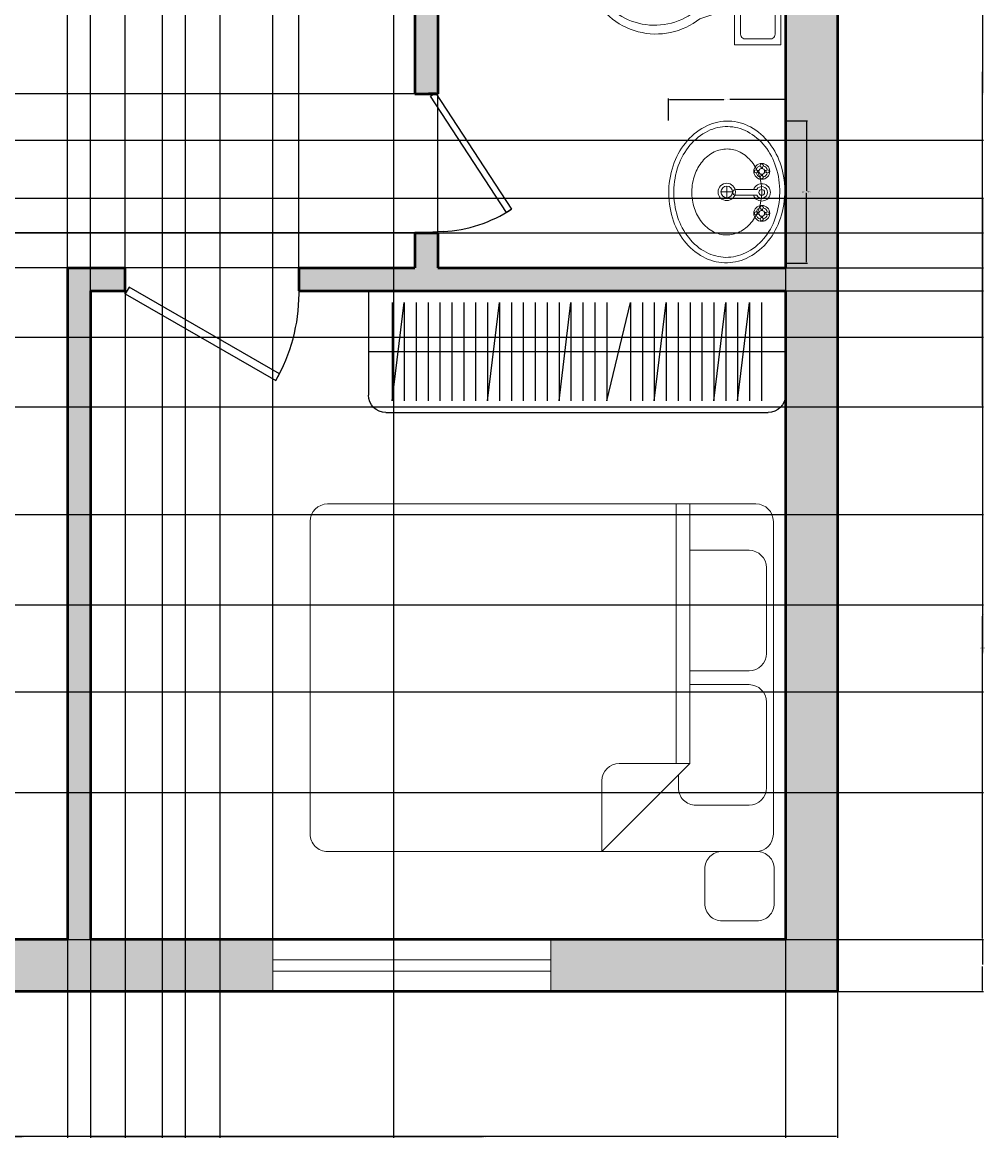
# Model space of a CAD drawing. Units: inches. Extents: x 3439 to 3988, y 1915 to 2284.
# Tile 5 of 7: x 3822 to 3988, y 1915 to 2108. Entities that reach past the tile are written whole.
import ezdxf

# ---------------------------------------------------------------- set-up
doc = ezdxf.new("R2010")
doc.units = ezdxf.units.IN
for name, color, linetype, lineweight in [('A-ANNO-DIMS', 2, 'Continuous', 18), ('A-DOOR', 3, 'Continuous', 25), ('A-FLOR-CASE', 8, 'Continuous', 25), ('A-FLOR-FIXT', 9, 'Continuous', 18), ('A-FURN', 9, 'Continuous', 18), ('A-GLAZ', 4, 'Continuous', 18), ('A-WALL', 7, 'Continuous', 50)]:
    doc.layers.add(name, color=color, linetype=linetype, lineweight=lineweight)
doc.layers.add('A-WALL-PATT', color=18, linetype='Continuous', lineweight=13, true_color=0x000000)
doc.styles.get("Standard").update_dxf_attribs({"font": 'arial.ttf'})
doc.dimstyles.get("Standard").update_dxf_attribs({"dimtxt": 0.18, "dimasz": 0.18, "dimexe": 0.18, "dimexo": 0.0625, "dimgap": 0.09, "dimtad": 0, "dimtih": 1, "dimtoh": 1, "dimdec": 4, "dimzin": 0, "dimdsep": 46, "dimtxsty": 'Standard', "dimcen": 0.09, "dimadec": 0, "dimazin": 0, "dimtfac": 1, "dimtdec": 4, "dimtofl": 0, "dimtmove": 0, "dimatfit": 3, "dimfxl": 1, "dimtolj": 1, "dimtzin": 0, "dimarcsym": 0})

# ---------------------------------------------------------------- blocks, each defined once
blk = doc.blocks.new('*U5')
for p, q in [((0, 0), (0, 6)), ((40, 0), (40, 6))]:
    blk.add_line(p, q)
blk.add_lwpolyline([(0, 0), (34.64, -20), (35.52, -18.48), (0.87, 1.52)], close=True)
blk.add_arc((0, 0), 40, 330, 0)
blk = doc.blocks.new('*U4')
for p, q in [((0, 0), (0, -6)), ((40, 0), (40, -6))]:
    blk.add_line(p, q)
blk.add_lwpolyline([(0, 0), (34.64, 20), (35.52, 18.48), (0.87, -1.52)], close=True)
blk.add_arc((0, 0), 40, 0, 30)
blk = doc.blocks.new('Toilet - top')
for p, q in [((9.5, -6), (9.5, -2)), ((-10, -8.5), (-8, -8.5)), ((-10, -9.5), (-10, -8.5)), ((-7, -9.5), (-10, -9.5)), ((-8, -8.5), (-8, -8)), ((-7, -8), (-7, -9.5)), ((-4, -8), (-6, -14)), ((4, -8), (6, -14)), ((4, -14), (-4, -14))]:
    blk.add_line(p, q)
blk.add_lwpolyline([(10.5, -8), (10.5, 0), (-10.5, 0), (-10.5, -8)], close=True)
for points in [[(8.5, -1), (-8.5, -1)], [(-9.5, -2), (-9.5, -6)], [(-8.5, -7), (8.5, -7)]]:
    blk.add_lwpolyline(points)
for centre, radius, start, end in [((-8.62, -1.88), 0.884, 81.8699, 188.1301), ((8.62, -1.88), 0.884, 351.8699, 98.1301), ((-8.62, -6.12), 0.884, 171.8699, 278.1301), ((8.62, -6.12), 0.884, 261.8699, 8.1301), ((3.52, -21.58), 12.17, 141.4691, 247.9714), ((4.2, -21.82), 11.33, 136.3677, 238.9468), ((-3.52, -21.58), 12.17, 292.0284, 38.5307), ((-4.2, -21.82), 11.33, 301.053, 43.6321), ((0, -27.88), 4, 245.7318, 294.2682), ((0, -29), 4, 254.8605, 285.1395)]:
    blk.add_arc(centre, radius, start, end)
blk = doc.blocks.new('Bed - Queen')
for p, q in [((3, 0), (56.99999, 0)), ((10.99999, -1.2), (25.79998, -1.2)), ((34.19999, -1.2), (48.99999, -1.2)), ((0, -77.00003), (0, -3)), ((59.99999, -3), (59.99999, -77.00003)), ((7.99999, -14.4), (7.99999, -4.2)), ((28.79998, -4.2), (28.79998, -14.4)), ((31.19999, -14.4), (31.19999, -4.2)), ((51.99999, -4.2), (51.99999, -13.4)), ((0, -14.4), (44.8, -14.4)), ((59.99999, -29.6), (44.8, -14.4)), ((44.8, -14.4), (44.8, -26.6)), ((44.8, -16.8), (0, -16.8)), ((48.99999, -16.4), (46.79936, -16.4)), ((47.8, -29.6), (59.99999, -29.6)), ((56.99999, -80.00003), (3, -80.00003))]:
    blk.add_line(p, q)
for centre, start, end in [((3, -3), 90, 180), ((56.99999, -3), 0, 90), ((10.99999, -4.2), 90, 180), ((25.79998, -4.2), 0, 90), ((34.19999, -4.2), 90, 180), ((48.99999, -4.2), 0, 90), ((48.99999, -13.4), 270, 0), ((47.8, -26.6), 180, 270), ((3, -77.00003), 180, 270), ((56.99999, -77.00003), 270, 0)]:
    blk.add_arc(centre, 3, start, end)
blk = doc.blocks.new('Sink - Oval top')
for p, q in [((-1, 0), (1, 0)), ((0, 1), (0, -1))]:
    blk.add_line(p, q)
for points in [[(-12.23, 0.39, 0.117634), (-11.46, -3.36, 0.104469), (-8.88, -6.8, 0.090016), (-5.08, -9.07, 0.08192), (-0.32, -10.02, 0.08192), (4.49, -9.38, 0.090016), (8.42, -7.36, 0.104469), (11.22, -4.09, 0.117634), (12.23, -0.39, 0.117634), (11.46, 3.36, 0.104469), (8.88, 6.8, 0.090016), (5.08, 9.07, 0.08192), (0.32, 10.02, 0.08192), (-4.49, 9.38, 0.090016), (-8.42, 7.36, 0.104469), (-11.22, 4.09, 0.117634)], [(-11.29, 0.16, 0.118622), (-10.52, -3.25, 0.104678), (-8.07, -6.36, 0.089562), (-4.54, -8.37, 0.081185), (-0.13, -9.15, 0.081185), (4.3, -8.49, 0.089562), (7.89, -6.58, 0.104678), (10.42, -3.55, 0.118622), (11.29, -0.16, 0.118622), (10.52, 3.25, 0.104678), (8.07, 6.36, 0.089562), (4.54, 8.37, 0.081185), (0.13, 9.15, 0.081185), (-4.3, 8.49, 0.089562), (-7.89, 6.58, 0.104678), (-10.42, 3.55, 0.118622)], [(-7.42, 0.08, 0.118283), (-6.91, -2.17, 0.104607), (-5.29, -4.21, 0.089718), (-2.97, -5.53, 0.081436), (-0.07, -6.04, 0.081436), (2.84, -5.59, 0.089718), (5.2, -4.33, 0.104607), (6.86, -2.32, 0.118283), (7.42, -0.08, 0.118283), (6.91, 2.17, 0.104607), (5.29, 4.21, 0.089718), (2.97, 5.53, 0.081436), (0.07, 6.04, 0.081436), (-2.84, 5.59, 0.089718), (-5.2, 4.33, 0.104607), (-6.86, 2.32, 0.118283)]]:
    blk.add_lwpolyline(points, format="xyb", close=True)
for radius in [1.5, 1]:
    blk.add_circle((0, 0), radius)
blk = doc.blocks.new('Faucet - Bathroom top')
for p, q in [((-4.107, 0.125), (-4.375, 0.125)), ((-3.75, 0.4788), (-3.75, 0.75)), ((-3.5, 0.482), (-3.5, 0.75)), ((-3.1461, 0.125), (-2.875, 0.125)), ((3.143, 0.125), (2.875, 0.125)), ((3.5, 0.4788), (3.5, 0.75)), ((3.75, 0.482), (3.75, 0.75)), ((4.1039, 0.125), (4.375, 0.125)), ((-4.1039, -0.125), (-4.375, -0.125)), ((-3.75, -0.4821), (-3.75, -0.75)), ((-3.5, -0.4789), (-3.5, -0.75)), ((-3.143, -0.125), (-2.875, -0.125)), ((-0.5, -0.8639), (-0.5, -4.5)), ((0.5, -4.5), (0.5, -0.8631)), ((3.1461, -0.125), (2.875, -0.125)), ((3.5, -0.4821), (3.5, -0.75)), ((3.75, -0.4789), (3.75, -0.75)), ((4.107, -0.125), (4.375, -0.125))]:
    blk.add_line(p, q)
for centre, radius in [((-3.625, 0), 1.375), ((-4.625, 0), 0.2795), ((-3.625, 0), 0.5), ((-3.625, 1), 0.2795), ((-2.625, 0), 0.2795), ((0, 0), 0.5), ((3.625, 0), 1.375), ((2.625, 0), 0.2795), ((3.625, 0), 0.5), ((3.625, 1), 0.2795), ((4.625, 0), 0.2795), ((-3.625, -1), 0.2795), ((3.625, -1), 0.2795)]:
    blk.add_circle(centre, radius)
for centre, radius, start, end in [((-3.625, 0), 1, 105.2407, 164.2093), ((-3.625, 0), 1, 16.44125, 74.07887), ((0, 0), 1.5, 289.6514, 250.3603), ((0, 0), 1, 300.3431, 239.7554), ((3.625, 0), 1, 106.12, 164.0884), ((3.625, 0), 1, 16.23422, 73.90469), ((-3.625, 0), 1, 196.2342, 253.9047), ((-3.625, 0), 1, 286.12, 344.0884), ((3.625, 0), 1, 196.4413, 254.0789), ((3.625, 0), 1, 285.2407, 344.2093), ((0, -4.5), 0.5, 180, 0)]:
    blk.add_arc(centre, radius, start, end)
blk = doc.blocks.new('WINDOW-GLASS-48IN')
for p, q in [((0, 2), (48, 2)), ((0, 0), (48, 0))]:
    blk.add_line(p, q)
blk = doc.blocks.new('WARDROBE-72IN')
for p, q in [((3, 21), (69, 21)), ((0, 0), (0, 18)), ((4.11, 2), (4.11, 19)), ((4.11, 19), (6.17, 2)), ((6.17, 2), (6.17, 19)), ((8.23, 2), (8.23, 19)), ((10.28, 2), (10.28, 19)), ((12.34, 2), (12.34, 19)), ((14.4, 2), (14.4, 19)), ((16.45, 2), (16.45, 19)), ((18.51, 2), (18.51, 19)), ((20.57, 2), (20.57, 19)), ((20.57, 19), (22.62, 2)), ((22.62, 2), (22.62, 19)), ((24.68, 2), (24.68, 19)), ((26.74, 2), (26.74, 19)), ((28.79, 2), (28.79, 19)), ((30.85, 2), (30.85, 19)), ((32.91, 2), (32.91, 19)), ((32.91, 19), (34.97, 2)), ((34.97, 2), (34.97, 19)), ((37.02, 2), (37.02, 19)), ((39.08, 2), (39.08, 19)), ((41.14, 2), (41.14, 19)), ((41.14, 19), (45.25, 2)), ((45.25, 2), (45.25, 19)), ((47.31, 2), (47.31, 19)), ((49.36, 2), (49.36, 19)), ((49.36, 19), (51.42, 2)), ((51.42, 2), (51.42, 19)), ((53.48, 2), (53.48, 19)), ((55.53, 2), (55.53, 19)), ((57.59, 2), (57.59, 19)), ((59.65, 2), (59.65, 19)), ((59.65, 19), (61.7, 2)), ((61.7, 2), (61.7, 19)), ((63.76, 2), (63.76, 19)), ((63.76, 19), (65.82, 2)), ((65.82, 2), (65.82, 19)), ((67.87, 2), (67.87, 19)), ((72, 18), (72, 0)), ((0, 10.5), (72, 10.5)), ((72, 0), (0, 0))]:
    blk.add_line(p, q)
for centre, start, end in [((3, 18), 90, 180), ((69, 18), 0, 90)]:
    blk.add_arc(centre, 3, start, end)
blk = doc.blocks.new('NIGHTSTAND-12IN-RADIUS')
blk.add_lwpolyline([(3, 0), (9, 0, 0.414214), (12, 3), (12, 9, 0.414214), (9, 12), (3, 12, 0.414214), (0, 9), (0, 3, 0.414214)], format="xyb", close=True)
blk = doc.blocks.new('*D33')
at = {"layer": 'A-ANNO-DIMS', "color": 0, "lineweight": -2, "transparency": 16777216}
for p, q in [((3953.59, 2090.71), (3957.39, 2090.71)), ((3957.21, 2090.53), (3957.21, 2078.62)), ((3957.21, 2066.34), (3957.21, 2078.25)), ((3953.59, 2066.16), (3957.39, 2066.16))]:
    blk.add_line(p, q, dxfattribs=at)
at = {"layer": 'A-ANNO-DIMS', "color": 0, "transparency": 16777216}
for points in [[(3957.18, 2090.53), (3957.24, 2090.53), (3957.21, 2090.71)], [(3957.18, 2066.34), (3957.24, 2066.34), (3957.21, 2066.16)]]:
    blk.add_solid(points, dxfattribs=at)
at = {"layer": 'Defpoints', "color": 0, "transparency": 16777216}
for p in [(3953.53, 2090.71), (3953.53, 2066.16), (3957.21, 2066.16)]:
    blk.add_point(p, dxfattribs=at)
at = {"layer": 'A-ANNO-DIMS', "color": 0, "transparency": 16777216, "insert": (3957.21, 2078.43), "char_height": 0.18, "attachment_point": 5}
blk.add_mtext('\\A1;BASIN 25 TYP.', dxfattribs=at)
blk = doc.blocks.new('*D34')
at = {"layer": 'A-ANNO-DIMS', "color": 0, "lineweight": -2, "transparency": 16777216}
for p, q in [((3933.4, 2090.77), (3933.4, 2094.57)), ((3933.58, 2094.39), (3942.93, 2094.39)), ((3953.35, 2094.39), (3943.99, 2094.39)), ((3953.53, 2090.77), (3953.53, 2094.57))]:
    blk.add_line(p, q, dxfattribs=at)
at = {"layer": 'A-ANNO-DIMS', "color": 0, "transparency": 16777216}
for points in [[(3933.58, 2094.42), (3933.58, 2094.36), (3933.4, 2094.39)], [(3953.35, 2094.42), (3953.35, 2094.36), (3953.53, 2094.39)]]:
    blk.add_solid(points, dxfattribs=at)
at = {"layer": 'Defpoints', "color": 0, "transparency": 16777216}
for p in [(3953.53, 2094.39), (3933.4, 2090.71), (3953.53, 2090.71)]:
    blk.add_point(p, dxfattribs=at)
at = {"layer": 'A-ANNO-DIMS', "color": 0, "transparency": 16777216, "insert": (3943.46, 2094.39), "char_height": 0.18, "attachment_point": 5}
blk.add_mtext('\\A1;20 TYP.', dxfattribs=at)
blk = doc.blocks.new('*D45')
at = {"layer": 'A-ANNO-DIMS', "color": 0, "lineweight": -2, "transparency": 16777216}
for p, q in [((3464.58, 1940.3), (3464.58, 1915.13)), ((3962.58, 1940.3), (3962.58, 1915.13)), ((3464.76, 1915.31), (3713.29, 1915.31)), ((3962.4, 1915.31), (3713.87, 1915.31))]:
    blk.add_line(p, q, dxfattribs=at)
at = {"layer": 'A-ANNO-DIMS', "color": 0, "transparency": 16777216}
for points in [[(3464.76, 1915.34), (3464.76, 1915.28), (3464.58, 1915.31)], [(3962.4, 1915.34), (3962.4, 1915.28), (3962.58, 1915.31)]]:
    blk.add_solid(points, dxfattribs=at)
at = {"layer": 'Defpoints', "color": 0, "transparency": 16777216}
for p in [(3464.58, 1940.36), (3962.58, 1940.36), (3962.58, 1915.31)]:
    blk.add_point(p, dxfattribs=at)
at = {"layer": 'A-ANNO-DIMS', "color": 0, "transparency": 16777216, "insert": (3713.58, 1915.31), "char_height": 0.18, "attachment_point": 5}
blk.add_mtext('\\A1;498', dxfattribs=at)
blk = doc.blocks.new('*D50')
at = {"layer": 'A-ANNO-DIMS', "color": 0, "lineweight": -2, "transparency": 16777216}
for p, q in [((3797.93, 2249.3), (3797.93, 1915.13)), ((3845.93, 2249.3), (3845.93, 1915.13)), ((3798.11, 1915.31), (3821.71, 1915.31)), ((3845.75, 1915.31), (3822.15, 1915.31))]:
    blk.add_line(p, q, dxfattribs=at)
at = {"layer": 'A-ANNO-DIMS', "color": 0, "transparency": 16777216}
for points in [[(3798.11, 1915.34), (3798.11, 1915.28), (3797.93, 1915.31)], [(3845.75, 1915.34), (3845.75, 1915.28), (3845.93, 1915.31)]]:
    blk.add_solid(points, dxfattribs=at)
at = {"layer": 'Defpoints', "color": 0, "transparency": 16777216}
for p in [(3797.93, 2249.36), (3845.93, 2249.36), (3845.93, 1915.31)]:
    blk.add_point(p, dxfattribs=at)
at = {"layer": 'A-ANNO-DIMS', "color": 0, "transparency": 16777216, "insert": (3821.93, 1915.31), "char_height": 0.18, "attachment_point": 5}
blk.add_mtext('\\A1;48', dxfattribs=at)
blk = doc.blocks.new('*D51')
at = {"layer": 'A-ANNO-DIMS', "color": 0, "lineweight": -2, "transparency": 16777216}
for p, q in [((3849.93, 2249.3), (3849.93, 1915.13)), ((3953.58, 2249.3), (3953.58, 1915.13)), ((3850.11, 1915.31), (3901.3, 1915.31)), ((3953.4, 1915.31), (3902.21, 1915.31))]:
    blk.add_line(p, q, dxfattribs=at)
at = {"layer": 'A-ANNO-DIMS', "color": 0, "transparency": 16777216}
for points in [[(3850.11, 1915.34), (3850.11, 1915.28), (3849.93, 1915.31)], [(3953.4, 1915.34), (3953.4, 1915.28), (3953.58, 1915.31)]]:
    blk.add_solid(points, dxfattribs=at)
at = {"layer": 'Defpoints', "color": 0, "transparency": 16777216}
for p in [(3849.93, 2249.36), (3953.58, 2249.36), (3953.58, 1915.31)]:
    blk.add_point(p, dxfattribs=at)
at = {"layer": 'A-ANNO-DIMS', "color": 0, "transparency": 16777216, "insert": (3901.76, 1915.31), "char_height": 0.18, "attachment_point": 5}
blk.add_mtext('\\A1;103.65', dxfattribs=at)
blk = doc.blocks.new('*D53')
at = {"layer": 'A-ANNO-DIMS', "color": 0, "lineweight": -2, "transparency": 16777216}
for p, q in [((3829.58, 2065.3), (3829.58, 1915.13)), ((3657.58, 2041.3), (3657.58, 1915.13)), ((3657.76, 1915.31), (3743.3, 1915.31)), ((3829.4, 1915.31), (3743.86, 1915.31))]:
    blk.add_line(p, q, dxfattribs=at)
at = {"layer": 'A-ANNO-DIMS', "color": 0, "transparency": 16777216}
for points in [[(3657.76, 1915.34), (3657.76, 1915.28), (3657.58, 1915.31)], [(3829.4, 1915.34), (3829.4, 1915.28), (3829.58, 1915.31)]]:
    blk.add_solid(points, dxfattribs=at)
at = {"layer": 'Defpoints', "color": 0, "transparency": 16777216}
for p in [(3829.58, 2065.36), (3657.58, 2041.36), (3829.58, 1915.31)]:
    blk.add_point(p, dxfattribs=at)
at = {"layer": 'A-ANNO-DIMS', "color": 0, "transparency": 16777216, "insert": (3743.58, 1915.31), "char_height": 0.18, "attachment_point": 5}
blk.add_mtext('\\A1;172', dxfattribs=at)
blk = doc.blocks.new('*D54')
at = {"layer": 'A-ANNO-DIMS', "color": 0, "lineweight": -2, "transparency": 16777216}
for p, q in [((3833.58, 1949.3), (3833.58, 1915.13)), ((3953.58, 1949.3), (3953.58, 1915.13)), ((3833.76, 1915.31), (3893.3, 1915.31)), ((3953.4, 1915.31), (3893.86, 1915.31))]:
    blk.add_line(p, q, dxfattribs=at)
at = {"layer": 'A-ANNO-DIMS', "color": 0, "transparency": 16777216}
for points in [[(3833.76, 1915.34), (3833.76, 1915.28), (3833.58, 1915.31)], [(3953.4, 1915.34), (3953.4, 1915.28), (3953.58, 1915.31)]]:
    blk.add_solid(points, dxfattribs=at)
at = {"layer": 'Defpoints', "color": 0, "transparency": 16777216}
for p in [(3833.58, 1949.36), (3953.58, 1949.36), (3953.58, 1915.31)]:
    blk.add_point(p, dxfattribs=at)
at = {"layer": 'A-ANNO-DIMS', "color": 0, "transparency": 16777216, "insert": (3893.58, 1915.31), "char_height": 0.18, "attachment_point": 5}
blk.add_mtext('\\A1;120', dxfattribs=at)
blk = doc.blocks.new('*D59')
at = {"layer": 'A-ANNO-DIMS', "color": 0, "lineweight": -2, "transparency": 16777216}
for p, q in [((3953.64, 2125.36), (3987.81, 2125.36)), ((3987.63, 2125.18), (3987.63, 2095.54)), ((3987.63, 2065.54), (3987.63, 2095.18)), ((3953.64, 2065.36), (3987.81, 2065.36))]:
    blk.add_line(p, q, dxfattribs=at)
at = {"layer": 'A-ANNO-DIMS', "color": 0, "transparency": 16777216}
for points in [[(3987.6, 2125.18), (3987.66, 2125.18), (3987.63, 2125.36)], [(3987.6, 2065.54), (3987.66, 2065.54), (3987.63, 2065.36)]]:
    blk.add_solid(points, dxfattribs=at)
at = {"layer": 'Defpoints', "color": 0, "transparency": 16777216}
for p in [(3953.58, 2125.36), (3987.63, 2125.36), (3953.58, 2065.36)]:
    blk.add_point(p, dxfattribs=at)
at = {"layer": 'A-ANNO-DIMS', "color": 0, "transparency": 16777216, "insert": (3987.63, 2095.36), "char_height": 0.18, "attachment_point": 5}
blk.add_mtext('\\A1;60', dxfattribs=at)
blk = doc.blocks.new('*D60')
at = {"layer": 'A-ANNO-DIMS', "color": 0, "lineweight": -2, "transparency": 16777216}
for p, q in [((3953.64, 2061.36), (3987.81, 2061.36)), ((3987.63, 2061.18), (3987.63, 2005.54)), ((3987.63, 1949.54), (3987.63, 2005.18)), ((3953.64, 1949.36), (3987.81, 1949.36))]:
    blk.add_line(p, q, dxfattribs=at)
at = {"layer": 'A-ANNO-DIMS', "color": 0, "transparency": 16777216}
for points in [[(3987.6, 2061.18), (3987.66, 2061.18), (3987.63, 2061.36)], [(3987.6, 1949.54), (3987.66, 1949.54), (3987.63, 1949.36)]]:
    blk.add_solid(points, dxfattribs=at)
at = {"layer": 'Defpoints', "color": 0, "transparency": 16777216}
for p in [(3953.58, 2061.36), (3987.63, 2061.36), (3953.58, 1949.36)]:
    blk.add_point(p, dxfattribs=at)
at = {"layer": 'A-ANNO-DIMS', "color": 0, "transparency": 16777216, "insert": (3987.63, 2005.36), "char_height": 0.18, "attachment_point": 5}
blk.add_mtext('\\A1;112', dxfattribs=at)
blk = doc.blocks.new('*D62')
at = {"layer": 'A-ANNO-DIMS', "color": 0, "lineweight": -2, "transparency": 16777216}
for p, q in [((3537.64, 2077.36), (3987.81, 2077.36)), ((3987.63, 2077.18), (3987.63, 2065.54)), ((3987.63, 2053.54), (3987.63, 2065.18)), ((3537.64, 2053.36), (3987.81, 2053.36))]:
    blk.add_line(p, q, dxfattribs=at)
at = {"layer": 'A-ANNO-DIMS', "color": 0, "transparency": 16777216}
for points in [[(3987.6, 2077.18), (3987.66, 2077.18), (3987.63, 2077.36)], [(3987.6, 2053.54), (3987.66, 2053.54), (3987.63, 2053.36)]]:
    blk.add_solid(points, dxfattribs=at)
at = {"layer": 'Defpoints', "color": 0, "transparency": 16777216}
for p in [(3537.58, 2077.36), (3987.63, 2077.36), (3537.58, 2053.36)]:
    blk.add_point(p, dxfattribs=at)
at = {"layer": 'A-ANNO-DIMS', "color": 0, "transparency": 16777216, "insert": (3987.63, 2065.36), "char_height": 0.18, "attachment_point": 5}
blk.add_mtext('\\A1;24', dxfattribs=at)
blk = doc.blocks.new('*D63')
at = {"layer": 'A-ANNO-DIMS', "color": 0, "lineweight": -2, "transparency": 16777216}
for p, q in [((3893.58, 2065.42), (3893.58, 2284)), ((3893.76, 2283.82), (3923.36, 2283.82)), ((3953.4, 2283.82), (3923.8, 2283.82)), ((3953.58, 2065.42), (3953.58, 2284))]:
    blk.add_line(p, q, dxfattribs=at)
at = {"layer": 'A-ANNO-DIMS', "color": 0, "transparency": 16777216}
for points in [[(3893.76, 2283.85), (3893.76, 2283.79), (3893.58, 2283.82)], [(3953.4, 2283.85), (3953.4, 2283.79), (3953.58, 2283.82)]]:
    blk.add_solid(points, dxfattribs=at)
at = {"layer": 'Defpoints', "color": 0, "transparency": 16777216}
for p in [(3953.58, 2283.82), (3893.58, 2065.36), (3953.58, 2065.36)]:
    blk.add_point(p, dxfattribs=at)
at = {"layer": 'A-ANNO-DIMS', "color": 0, "transparency": 16777216, "insert": (3923.58, 2283.82), "char_height": 0.18, "attachment_point": 5}
blk.add_mtext('\\A1;60', dxfattribs=at)
blk = doc.blocks.new('*D76')
at = {"layer": 'A-ANNO-DIMS', "color": 0, "lineweight": -2, "transparency": 16777216}
for p, q in [((3833.58, 1949.42), (3833.58, 2284)), ((3833.76, 2283.82), (3849.01, 2283.82)), ((3864.9, 2283.82), (3849.66, 2283.82)), ((3865.08, 1949.42), (3865.08, 2284))]:
    blk.add_line(p, q, dxfattribs=at)
at = {"layer": 'A-ANNO-DIMS', "color": 0, "transparency": 16777216}
for points in [[(3833.76, 2283.85), (3833.76, 2283.79), (3833.58, 2283.82)], [(3864.9, 2283.85), (3864.9, 2283.79), (3865.08, 2283.82)]]:
    blk.add_solid(points, dxfattribs=at)
at = {"layer": 'Defpoints', "color": 0, "transparency": 16777216}
for p in [(3865.08, 2283.82), (3833.58, 1949.36), (3865.08, 1949.36)]:
    blk.add_point(p, dxfattribs=at)
at = {"layer": 'A-ANNO-DIMS', "color": 0, "transparency": 16777216, "insert": (3849.33, 2283.82), "char_height": 0.18, "attachment_point": 5}
blk.add_mtext('\\A1;31.5', dxfattribs=at)
blk = doc.blocks.new('*D83')
at = {"layer": 'A-ANNO-DIMS', "color": 0, "lineweight": -2, "transparency": 16777216}
for p, q in [((3537.64, 2111.36), (3987.81, 2111.36)), ((3987.63, 2111.18), (3987.63, 2099.54)), ((3987.63, 2087.54), (3987.63, 2099.18)), ((3537.64, 2087.36), (3987.81, 2087.36))]:
    blk.add_line(p, q, dxfattribs=at)
at = {"layer": 'A-ANNO-DIMS', "color": 0, "transparency": 16777216}
for points in [[(3987.6, 2111.18), (3987.66, 2111.18), (3987.63, 2111.36)], [(3987.6, 2087.54), (3987.66, 2087.54), (3987.63, 2087.36)]]:
    blk.add_solid(points, dxfattribs=at)
at = {"layer": 'Defpoints', "color": 0, "transparency": 16777216}
for p in [(3537.58, 2111.36), (3987.63, 2111.36), (3537.58, 2087.36)]:
    blk.add_point(p, dxfattribs=at)
at = {"layer": 'A-ANNO-DIMS', "color": 0, "transparency": 16777216, "insert": (3987.63, 2099.36), "char_height": 0.18, "attachment_point": 5}
blk.add_mtext('\\A1;24', dxfattribs=at)
blk = doc.blocks.new('*D85')
at = {"layer": 'A-ANNO-DIMS', "color": 0, "lineweight": -2, "transparency": 16777216}
for p, q in [((3855.93, 2125.3), (3855.93, 1915.13)), ((3885.93, 2125.3), (3885.93, 1915.13)), ((3856.11, 1915.31), (3870.71, 1915.31)), ((3885.75, 1915.31), (3871.15, 1915.31))]:
    blk.add_line(p, q, dxfattribs=at)
at = {"layer": 'A-ANNO-DIMS', "color": 0, "transparency": 16777216}
for points in [[(3856.11, 1915.34), (3856.11, 1915.28), (3855.93, 1915.31)], [(3885.75, 1915.34), (3885.75, 1915.28), (3885.93, 1915.31)]]:
    blk.add_solid(points, dxfattribs=at)
at = {"layer": 'Defpoints', "color": 0, "transparency": 16777216}
for p in [(3855.93, 2125.36), (3885.93, 2125.36), (3885.93, 1915.31)]:
    blk.add_point(p, dxfattribs=at)
at = {"layer": 'A-ANNO-DIMS', "color": 0, "transparency": 16777216, "insert": (3870.93, 1915.31), "char_height": 0.18, "attachment_point": 5}
blk.add_mtext('\\A1;30', dxfattribs=at)
blk = doc.blocks.new('*D86')
at = {"layer": 'A-ANNO-DIMS', "color": 0, "lineweight": -2, "transparency": 16777216}
for p, q in [((3833.58, 2061.3), (3833.58, 1915.13)), ((3839.58, 2061.3), (3839.58, 1915.13)), ((3833.76, 1915.31), (3836.43, 1915.31)), ((3839.4, 1915.31), (3836.73, 1915.31))]:
    blk.add_line(p, q, dxfattribs=at)
at = {"layer": 'A-ANNO-DIMS', "color": 0, "transparency": 16777216}
for points in [[(3833.76, 1915.34), (3833.76, 1915.28), (3833.58, 1915.31)], [(3839.4, 1915.34), (3839.4, 1915.28), (3839.58, 1915.31)]]:
    blk.add_solid(points, dxfattribs=at)
at = {"layer": 'Defpoints', "color": 0, "transparency": 16777216}
for p in [(3833.58, 2061.36), (3839.58, 2061.36), (3839.58, 1915.31)]:
    blk.add_point(p, dxfattribs=at)
at = {"layer": 'A-ANNO-DIMS', "color": 0, "transparency": 16777216, "insert": (3836.58, 1915.31), "char_height": 0.18, "attachment_point": 5}
blk.add_mtext('\\A1;6', dxfattribs=at)
blk = doc.blocks.new('*D87')
at = {"layer": 'A-ANNO-DIMS', "color": 0, "lineweight": -2, "transparency": 16777216}
for p, q in [((3839.58, 2065.42), (3839.58, 2284)), ((3839.76, 2283.82), (3854.36, 2283.82)), ((3869.4, 2283.82), (3854.8, 2283.82)), ((3869.58, 2065.42), (3869.58, 2284))]:
    blk.add_line(p, q, dxfattribs=at)
at = {"layer": 'A-ANNO-DIMS', "color": 0, "transparency": 16777216}
for points in [[(3839.76, 2283.85), (3839.76, 2283.79), (3839.58, 2283.82)], [(3869.4, 2283.85), (3869.4, 2283.79), (3869.58, 2283.82)]]:
    blk.add_solid(points, dxfattribs=at)
at = {"layer": 'Defpoints', "color": 0, "transparency": 16777216}
for p in [(3869.58, 2283.82), (3839.58, 2065.36), (3869.58, 2065.36)]:
    blk.add_point(p, dxfattribs=at)
at = {"layer": 'A-ANNO-DIMS', "color": 0, "transparency": 16777216, "insert": (3854.58, 2283.82), "char_height": 0.18, "attachment_point": 5}
blk.add_mtext('\\A1;30', dxfattribs=at)
blk = doc.blocks.new('*D88')
at = {"layer": 'A-ANNO-DIMS', "color": 0, "lineweight": -2, "transparency": 16777216}
for p, q in [((3653.64, 2077.36), (3987.81, 2077.36)), ((3987.63, 2077.18), (3987.63, 2074.54)), ((3987.63, 2071.54), (3987.63, 2074.18)), ((3653.64, 2071.36), (3987.81, 2071.36))]:
    blk.add_line(p, q, dxfattribs=at)
at = {"layer": 'A-ANNO-DIMS', "color": 0, "transparency": 16777216}
for points in [[(3987.6, 2077.18), (3987.66, 2077.18), (3987.63, 2077.36)], [(3987.6, 2071.54), (3987.66, 2071.54), (3987.63, 2071.36)]]:
    blk.add_solid(points, dxfattribs=at)
at = {"layer": 'Defpoints', "color": 0, "transparency": 16777216}
for p in [(3653.58, 2077.36), (3987.63, 2077.36), (3653.58, 2071.36)]:
    blk.add_point(p, dxfattribs=at)
at = {"layer": 'A-ANNO-DIMS', "color": 0, "transparency": 16777216, "insert": (3987.63, 2074.36), "char_height": 0.18, "attachment_point": 5}
blk.add_mtext('\\A1;6', dxfattribs=at)
blk = doc.blocks.new('*D89')
at = {"layer": 'A-ANNO-DIMS', "color": 0, "lineweight": -2, "transparency": 16777216}
for p, q in [((3657.64, 2071.36), (3987.81, 2071.36)), ((3987.63, 2071.18), (3987.63, 2056.54)), ((3987.63, 2041.54), (3987.63, 2056.18)), ((3657.64, 2041.36), (3987.81, 2041.36))]:
    blk.add_line(p, q, dxfattribs=at)
at = {"layer": 'A-ANNO-DIMS', "color": 0, "transparency": 16777216}
for points in [[(3987.6, 2071.18), (3987.66, 2071.18), (3987.63, 2071.36)], [(3987.6, 2041.54), (3987.66, 2041.54), (3987.63, 2041.36)]]:
    blk.add_solid(points, dxfattribs=at)
at = {"layer": 'Defpoints', "color": 0, "transparency": 16777216}
for p in [(3657.58, 2071.36), (3987.63, 2071.36), (3657.58, 2041.36)]:
    blk.add_point(p, dxfattribs=at)
at = {"layer": 'A-ANNO-DIMS', "color": 0, "transparency": 16777216, "insert": (3987.63, 2056.36), "char_height": 0.18, "attachment_point": 5}
blk.add_mtext('\\A1;30', dxfattribs=at)
blk = doc.blocks.new('*D90')
at = {"layer": 'A-ANNO-DIMS', "color": 0, "lineweight": -2, "transparency": 16777216}
for p, q in [((3889.52, 2071.36), (3439.35, 2071.36)), ((3439.53, 2071.18), (3439.53, 2068.54)), ((3439.53, 2065.54), (3439.53, 2068.18)), ((3889.52, 2065.36), (3439.35, 2065.36))]:
    blk.add_line(p, q, dxfattribs=at)
at = {"layer": 'A-ANNO-DIMS', "color": 0, "transparency": 16777216}
for points in [[(3439.5, 2071.18), (3439.56, 2071.18), (3439.53, 2071.36)], [(3439.5, 2065.54), (3439.56, 2065.54), (3439.53, 2065.36)]]:
    blk.add_solid(points, dxfattribs=at)
at = {"layer": 'Defpoints', "color": 0, "transparency": 16777216}
for p in [(3439.53, 2071.36), (3889.58, 2071.36), (3889.58, 2065.36)]:
    blk.add_point(p, dxfattribs=at)
at = {"layer": 'A-ANNO-DIMS', "color": 0, "transparency": 16777216, "insert": (3439.53, 2068.36), "char_height": 0.18, "attachment_point": 5}
blk.add_mtext('\\A1;6', dxfattribs=at)
blk = doc.blocks.new('*D91')
at = {"layer": 'A-ANNO-DIMS', "color": 0, "lineweight": -2, "transparency": 16777216}
for p, q in [((3889.52, 2095.36), (3439.35, 2095.36)), ((3439.53, 2095.18), (3439.53, 2083.54)), ((3439.53, 2071.54), (3439.53, 2083.18)), ((3889.52, 2071.36), (3439.35, 2071.36))]:
    blk.add_line(p, q, dxfattribs=at)
at = {"layer": 'A-ANNO-DIMS', "color": 0, "transparency": 16777216}
for points in [[(3439.5, 2095.18), (3439.56, 2095.18), (3439.53, 2095.36)], [(3439.5, 2071.54), (3439.56, 2071.54), (3439.53, 2071.36)]]:
    blk.add_solid(points, dxfattribs=at)
at = {"layer": 'Defpoints', "color": 0, "transparency": 16777216}
for p in [(3439.53, 2095.36), (3889.58, 2095.36), (3889.58, 2071.36)]:
    blk.add_point(p, dxfattribs=at)
at = {"layer": 'A-ANNO-DIMS', "color": 0, "transparency": 16777216, "insert": (3439.53, 2083.36), "char_height": 0.18, "attachment_point": 5}
blk.add_mtext('\\A1;24', dxfattribs=at)
blk = doc.blocks.new('*D92')
at = {"layer": 'A-ANNO-DIMS', "color": 0, "lineweight": -2, "transparency": 16777216}
for p, q in [((3767.64, 1949.36), (3987.81, 1949.36)), ((3987.63, 1949.18), (3987.63, 1945.04)), ((3987.63, 1940.54), (3987.63, 1944.68)), ((3767.64, 1940.36), (3987.81, 1940.36))]:
    blk.add_line(p, q, dxfattribs=at)
at = {"layer": 'A-ANNO-DIMS', "color": 0, "transparency": 16777216}
for points in [[(3987.6, 1949.18), (3987.66, 1949.18), (3987.63, 1949.36)], [(3987.6, 1940.54), (3987.66, 1940.54), (3987.63, 1940.36)]]:
    blk.add_solid(points, dxfattribs=at)
at = {"layer": 'Defpoints', "color": 0, "transparency": 16777216}
for p in [(3767.58, 1949.36), (3987.63, 1949.36), (3767.58, 1940.36)]:
    blk.add_point(p, dxfattribs=at)
at = {"layer": 'A-ANNO-DIMS', "color": 0, "transparency": 16777216, "insert": (3987.63, 1944.86), "char_height": 0.18, "attachment_point": 5}
blk.add_mtext('\\A1;9', dxfattribs=at)
blk = doc.blocks.new('*D93')
at = {"layer": 'A-ANNO-DIMS', "color": 0, "lineweight": -2, "transparency": 16777216}
for p, q in [((3829.58, 2065.42), (3829.58, 2284)), ((3829.76, 2283.82), (3831.43, 2283.82)), ((3833.4, 2283.82), (3831.73, 2283.82)), ((3833.58, 2061.42), (3833.58, 2284))]:
    blk.add_line(p, q, dxfattribs=at)
at = {"layer": 'A-ANNO-DIMS', "color": 0, "transparency": 16777216}
for points in [[(3829.76, 2283.85), (3829.76, 2283.79), (3829.58, 2283.82)], [(3833.4, 2283.85), (3833.4, 2283.79), (3833.58, 2283.82)]]:
    blk.add_solid(points, dxfattribs=at)
at = {"layer": 'Defpoints', "color": 0, "transparency": 16777216}
for p in [(3833.58, 2283.82), (3829.58, 2065.36), (3833.58, 2061.36)]:
    blk.add_point(p, dxfattribs=at)
at = {"layer": 'A-ANNO-DIMS', "color": 0, "transparency": 16777216, "insert": (3831.58, 2283.82), "char_height": 0.18, "attachment_point": 5}
blk.add_mtext('\\A1;4', dxfattribs=at)
blk = doc.blocks.new('*D100')
at = {"layer": 'A-ANNO-DIMS', "color": 0, "lineweight": -2, "transparency": 16777216}
for p, q in [((3681.83, 2022.72), (3987.81, 2022.72)), ((3987.63, 2022.54), (3987.63, 1998.91)), ((3987.63, 1974.9), (3987.63, 1998.54)), ((3681.83, 1974.72), (3987.81, 1974.72))]:
    blk.add_line(p, q, dxfattribs=at)
at = {"layer": 'A-ANNO-DIMS', "color": 0, "transparency": 16777216}
for points in [[(3987.6, 2022.54), (3987.66, 2022.54), (3987.63, 2022.72)], [(3987.6, 1974.9), (3987.66, 1974.9), (3987.63, 1974.72)]]:
    blk.add_solid(points, dxfattribs=at)
at = {"layer": 'Defpoints', "color": 0, "transparency": 16777216}
for p in [(3681.76, 2022.72), (3987.63, 2022.72), (3681.76, 1974.72)]:
    blk.add_point(p, dxfattribs=at)
at = {"layer": 'A-ANNO-DIMS', "color": 0, "transparency": 16777216, "insert": (3987.63, 1998.72), "char_height": 0.18, "attachment_point": 5}
blk.add_mtext('\\A1;48', dxfattribs=at)
blk = doc.blocks.new('*D102')
at = {"layer": 'A-ANNO-DIMS', "color": 0, "lineweight": -2, "transparency": 16777216}
for p, q in [((3705.48, 2007.16), (3987.81, 2007.16)), ((3987.63, 2006.98), (3987.63, 1999.83)), ((3987.63, 1992.31), (3987.63, 1999.46)), ((3705.48, 1992.13), (3987.81, 1992.13))]:
    blk.add_line(p, q, dxfattribs=at)
at = {"layer": 'A-ANNO-DIMS', "color": 0, "transparency": 16777216}
for points in [[(3987.6, 2006.98), (3987.66, 2006.98), (3987.63, 2007.16)], [(3987.6, 1992.31), (3987.66, 1992.31), (3987.63, 1992.13)]]:
    blk.add_solid(points, dxfattribs=at)
at = {"layer": 'Defpoints', "color": 0, "transparency": 16777216}
for p in [(3705.42, 2007.16), (3987.63, 2007.16), (3705.42, 1992.13)]:
    blk.add_point(p, dxfattribs=at)
at = {"layer": 'A-ANNO-DIMS', "color": 0, "transparency": 16777216, "insert": (3987.63, 1999.64), "char_height": 0.18, "attachment_point": 5}
blk.add_mtext('\\A1;15.025', dxfattribs=at)

msp = doc.modelspace()

# ---------------------------------------------------------------- hatches: boundary and pattern name
at = {"layer": 'A-WALL-PATT'}
h = msp.add_hatch(color=256, dxfattribs=at)
h.dxf.hatch_style = 1
h.paths.add_polyline_path([(3962.5815, 2258.3617), (3929.3564, 2258.3617), (3929.3564, 2249.3617), (3953.5815, 2249.3617), (3953.5815, 2129.3617), (3885.9319, 2129.3617), (3885.9319, 2125.3617), (3889.5815, 2125.3617), (3889.5815, 2095.3617), (3893.5815, 2095.3617), (3893.5815, 2125.3617), (3953.5815, 2125.3617), (3953.5815, 2065.3617), (3893.5815, 2065.3617), (3893.5815, 2071.3617), (3889.5815, 2071.3617), (3889.5815, 2065.3617), (3869.5815, 2065.3617), (3869.5815, 2061.3617), (3953.5815, 2061.3617), (3953.5815, 1949.3617), (3913.0815, 1949.3617), (3913.0815, 1940.3617), (3962.5815, 1940.3617)])
h = msp.add_hatch(color=256, dxfattribs=at)
h.dxf.hatch_style = 1
h.paths.add_polyline_path([(3865.0815, 1949.3617), (3833.5815, 1949.3617), (3833.5815, 2061.3617), (3839.5815, 2061.3617), (3839.5815, 2065.3617), (3829.5815, 2065.3617), (3829.5815, 1949.3617), (3767.5815, 1949.3617), (3767.5815, 1940.3617), (3865.0815, 1940.3617)])

# ---------------------------------------------------------------- linework, layer by layer
at = {"layer": 'A-GLAZ'}
for points in [[(3865.0815, 1940.3617), (3865.0815, 1949.3617)], [(3913.0815, 1949.3617), (3913.0815, 1940.3617)]]:
    msp.add_lwpolyline(points, dxfattribs=at)
at = {"layer": 'A-WALL'}
for p, q in [((3889.5815, 2125.3617), (3889.5815, 2095.3617)), ((3893.5815, 2125.3617), (3893.5815, 2095.3617)), ((3953.5815, 2125.3617), (3953.5815, 2065.3617)), ((3889.5815, 2095.3617), (3893.5815, 2095.3617)), ((3889.5815, 2071.3617), (3893.5815, 2071.3617)), ((3889.5815, 2071.3617), (3889.5815, 2065.3617)), ((3893.5815, 2071.3617), (3893.5815, 2065.3617)), ((3829.5815, 2065.3617), (3839.5815, 2065.3617)), ((3829.5815, 2065.3617), (3829.5815, 1949.3617)), ((3839.5815, 2061.3617), (3839.5815, 2065.3617)), ((3869.5815, 2061.3617), (3869.5815, 2065.3617)), ((3869.5815, 2065.3617), (3889.5815, 2065.3617)), ((3893.5815, 2065.3617), (3953.5815, 2065.3617)), ((3833.5815, 2061.3617), (3839.5815, 2061.3617)), ((3833.5815, 2061.3617), (3833.5815, 1949.3617)), ((3869.5815, 2061.3617), (3953.5815, 2061.3617)), ((3953.5815, 2061.3617), (3953.5815, 1949.3617)), ((3829.5815, 1949.3617), (3767.5815, 1949.3617)), ((3953.5815, 1949.3617), (3833.5815, 1949.3617))]:
    msp.add_line(p, q, dxfattribs=at)
msp.add_lwpolyline([(3827.9319, 2258.3617), (3962.5815, 2258.3617), (3962.5815, 1940.3617), (3767.5815, 1940.3617)], dxfattribs=at)

# ---------------------------------------------------------------- block references
at = {"layer": 'A-DOOR', "xscale": 0.5999999999999998, "yscale": 0.5999999999999998, "zscale": 0.5999999999999998, "rotation": 273.1445926596106}
msp.add_blockref('*U4', (3893.1761, 2095.5592), dxfattribs=at)
at = {"layer": 'A-DOOR', "xscale": 0.75, "yscale": 0.75, "zscale": 0.75}
msp.add_blockref('*U5', (3839.5815, 2060.8617), dxfattribs=at)
at = {"layer": 'A-FLOR-CASE', "extrusion": (0, 0, -1), "zscale": -1, "rotation": 180}
msp.add_blockref('WARDROBE-72IN', (-3881.5815, 2061.3617), dxfattribs=at)
msp.add_blockref('WARDROBE-72IN', (-3881.5815, 2061.3617), dxfattribs=at)
at = {"layer": 'A-FLOR-FIXT', "rotation": 269.9999999999999}
for name, p in [('Toilet - top', (3952.8222, 2114.3538)), ('Sink - Oval top', (3943.4638, 2078.4325)), ('Faucet - Bathroom top', (3949.5007, 2078.365))]:
    msp.add_blockref(name, p, dxfattribs=at)
at = {"layer": 'A-FURN', "rotation": 270}
msp.add_blockref('Bed - Queen', (3951.5053, 2024.5575), dxfattribs=at)
at = {"layer": 'A-FURN'}
msp.add_blockref('NIGHTSTAND-12IN-RADIUS', (3939.662, 1952.5575), dxfattribs=at)
at = {"layer": 'A-GLAZ'}
msp.add_blockref('WINDOW-GLASS-48IN', (3865.0815, 1943.8617), dxfattribs=at)

# ---------------------------------------------------------------- dimensions: what is measured, and where the dimension line sits
at = {"layer": 'A-ANNO-DIMS'}
for base, p1, p2, override, picture, middle in [((3833.5815, 2283.8228), (3829.5815, 2065.3617), (3833.5815, 2061.3617), {"dimdec": 0, "dimlfac": 1, "dimrnd": 0, "dimzin": 0, "dimdsep": 46, "dimlunit": 2}, '*D93', (3831.5815, 2283.8228)), ((3865.0815, 2283.8228), (3833.5815, 1949.3617), (3865.0815, 1949.3617), {"dimdec": 1, "dimlfac": 1, "dimrnd": 0, "dimzin": 0, "dimdsep": 46, "dimlunit": 2}, '*D76', (3849.3315, 2283.8228)), ((3869.5815, 2283.8228), (3839.5815, 2065.3617), (3869.5815, 2065.3617), {"dimdec": 0, "dimlfac": 1, "dimrnd": 0, "dimzin": 0, "dimdsep": 46, "dimlunit": 2}, '*D87', (3854.5815, 2283.8228)), ((3953.5815, 2283.8228), (3893.5815, 2065.3617), (3953.5815, 2065.3617), {"dimdec": 0, "dimlfac": 1, "dimrnd": 0, "dimzin": 0, "dimdsep": 46, "dimlunit": 2}, '*D63', (3923.5815, 2283.8228)), ((3845.9319, 1915.3117), (3797.9319, 2249.3617), (3845.9319, 2249.3617), {"dimdec": 0, "dimlfac": 1, "dimrnd": 0, "dimzin": 0, "dimdsep": 46, "dimlunit": 2}, '*D50', (3821.9319, 1915.3117)), ((3953.5815, 1915.3117), (3849.9319, 2249.3617), (3953.5815, 2249.3617), {"dimdec": 2, "dimlfac": 1, "dimrnd": 0, "dimzin": 0, "dimdsep": 46, "dimlunit": 2}, '*D51', (3901.7567, 1915.3117)), ((3885.9319, 1915.3117), (3855.9319, 2125.3617), (3885.9319, 2125.3617), {"dimdec": 0, "dimlfac": 1, "dimrnd": 0, "dimzin": 0, "dimdsep": 46, "dimlunit": 2}, '*D85', (3870.9319, 1915.3117)), ((3829.5815, 1915.3117), (3657.5815, 2041.3617), (3829.5815, 2065.3617), {"dimdec": 0, "dimlfac": 1, "dimrnd": 0, "dimzin": 0, "dimdsep": 46, "dimlunit": 2}, '*D53', (3743.5815, 1915.3117)), ((3839.5815, 1915.3117), (3833.5815, 2061.3617), (3839.5815, 2061.3617), {"dimdec": 0, "dimlfac": 1, "dimrnd": 0, "dimzin": 0, "dimdsep": 46, "dimlunit": 2}, '*D86', (3836.5815, 1915.3117)), ((3953.5815, 1915.3117), (3833.5815, 1949.3617), (3953.5815, 1949.3617), {"dimdec": 0, "dimlfac": 1, "dimrnd": 0, "dimzin": 0, "dimdsep": 46, "dimlunit": 2}, '*D54', (3893.5815, 1915.3117)), ((3962.5815, 1915.3117), (3464.5815, 1940.3617), (3962.5815, 1940.3617), {"dimdec": 0, "dimlfac": 1, "dimrnd": 0, "dimzin": 0, "dimdsep": 46, "dimlunit": 2}, '*D45', (3713.5815, 1915.3117))]:
    dim = msp.add_linear_dim(base=base, p1=p1, p2=p2, dimstyle='Standard', override=override, dxfattribs=at)
    dim.commit()
    dim.dimension.update_dxf_attribs({"geometry": picture, "text_midpoint": middle})
for base, p1, p2, override, picture, middle in [((3987.6315, 2125.3617), (3953.5815, 2065.3617), (3953.5815, 2125.3617), {"dimdec": 0, "dimlfac": 1, "dimrnd": 0, "dimzin": 0, "dimdsep": 46, "dimlunit": 2}, '*D59', (3987.6315, 2095.3617)), ((3987.6315, 2111.3617), (3537.5815, 2087.3617), (3537.5815, 2111.3617), {"dimdec": 0, "dimlfac": 1, "dimrnd": 0, "dimzin": 0, "dimdsep": 46, "dimlunit": 2}, '*D83', (3987.6315, 2099.3617)), ((3439.5315, 2095.3617), (3889.5815, 2071.3617), (3889.5815, 2095.3617), {"dimdec": 0, "dimlfac": 1, "dimrnd": 0, "dimzin": 0, "dimdsep": 46, "dimlunit": 2}, '*D91', (3439.5315, 2083.3617)), ((3987.6315, 2077.3617), (3537.5815, 2053.3617), (3537.5815, 2077.3617), {"dimdec": 0, "dimlfac": 1, "dimrnd": 0, "dimzin": 0, "dimdsep": 46, "dimlunit": 2}, '*D62', (3987.6315, 2065.3617)), ((3987.6315, 2077.3617), (3653.5815, 2071.3617), (3653.5815, 2077.3617), {"dimdec": 0, "dimlfac": 1, "dimrnd": 0, "dimzin": 0, "dimdsep": 46, "dimlunit": 2}, '*D88', (3987.6315, 2074.3617)), ((3439.5315, 2071.3617), (3889.5815, 2065.3617), (3889.5815, 2071.3617), {"dimdec": 0, "dimlfac": 1, "dimrnd": 0, "dimzin": 0, "dimdsep": 46, "dimlunit": 2}, '*D90', (3439.5315, 2068.3617)), ((3987.6315, 2071.3617), (3657.5815, 2041.3617), (3657.5815, 2071.3617), {"dimdec": 0, "dimlfac": 1, "dimrnd": 0, "dimzin": 0, "dimdsep": 46, "dimlunit": 2}, '*D89', (3987.6315, 2056.3617)), ((3987.6315, 2061.3617), (3953.5815, 1949.3617), (3953.5815, 2061.3617), {"dimdec": 0, "dimlfac": 1, "dimrnd": 0, "dimzin": 0, "dimdsep": 46, "dimlunit": 2}, '*D60', (3987.6315, 2005.3617)), ((3987.6315, 2022.7238), (3681.7646, 1974.7238), (3681.7646, 2022.7238), {"dimdec": 0, "dimlfac": 1, "dimrnd": 0, "dimzin": 0, "dimdsep": 46, "dimlunit": 2}, '*D100', (3987.6315, 1998.7238)), ((3987.6315, 2007.1572), (3705.4216, 1992.1326), (3705.4216, 2007.1572), {"dimdec": 3, "dimlfac": 1, "dimrnd": 0, "dimzin": 0, "dimdsep": 46, "dimlunit": 2}, '*D102', (3987.6315, 1999.6449)), ((3987.6315, 1949.3617), (3767.5815, 1940.3617), (3767.5815, 1949.3617), {"dimdec": 0, "dimlfac": 1, "dimrnd": 0, "dimzin": 0, "dimdsep": 46, "dimlunit": 2}, '*D92', (3987.6315, 1944.8617))]:
    dim = msp.add_linear_dim(base=base, p1=p1, p2=p2, angle=90, dimstyle='Standard', override=override, dxfattribs=at)
    dim.commit()
    dim.dimension.update_dxf_attribs({"geometry": picture, "text_midpoint": middle})
dim = msp.add_linear_dim(base=(3953.5321, 2094.3906), p1=(3933.3956, 2090.708), p2=(3953.5321, 2090.708), text='<> TYP.', dimstyle='Standard', override={"dimdec": 0, "dimlfac": 1, "dimrnd": 0, "dimzin": 0, "dimdsep": 46, "dimlunit": 2}, dxfattribs=at)
dim.commit()
dim.dimension.update_dxf_attribs({"geometry": '*D34', "text_midpoint": (3943.4638, 2094.3906)})
dim = msp.add_linear_dim(base=(3957.2148, 2066.1571), p1=(3953.5321, 2090.708), p2=(3953.5321, 2066.1571), angle=270, text='BASIN <> TYP.', dimstyle='Standard', override={"dimdec": 0, "dimlfac": 1, "dimrnd": 0, "dimzin": 0, "dimdsep": 46, "dimlunit": 2}, dxfattribs=at)
dim.commit()
dim.dimension.update_dxf_attribs({"geometry": '*D33', "text_midpoint": (3957.2148, 2078.4325)})

doc.saveas('drawing.dxf')
